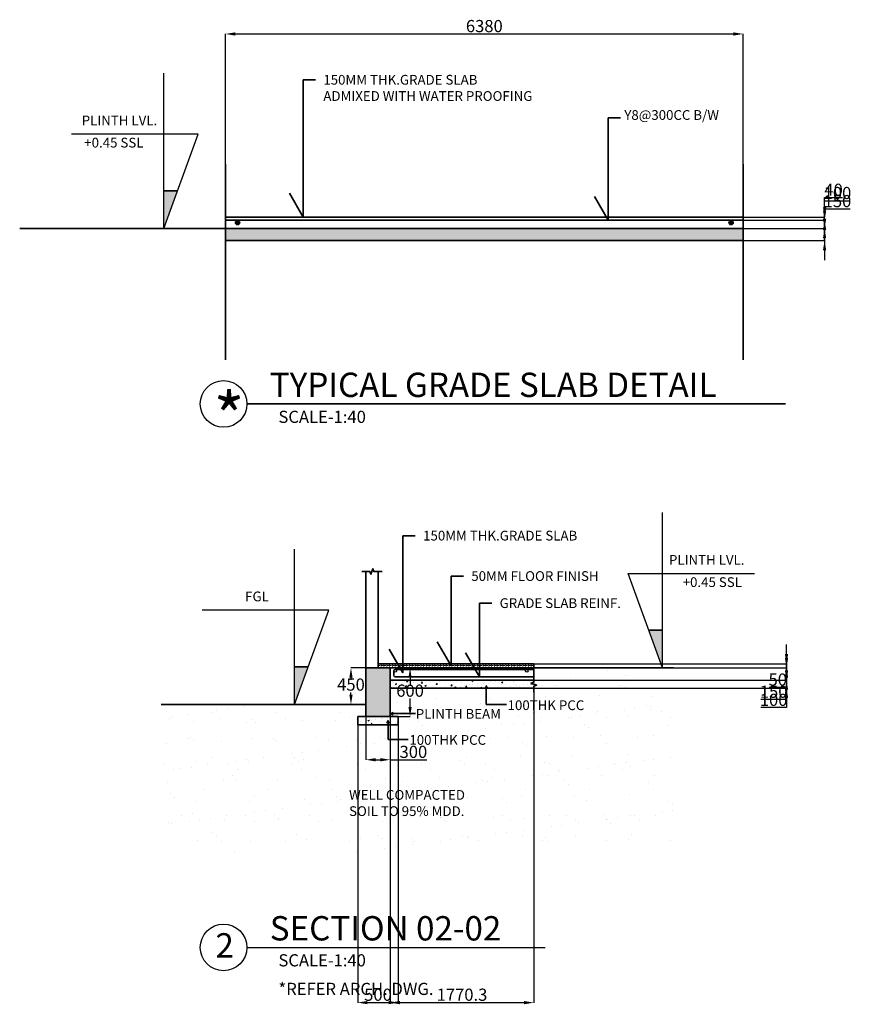
# Model space of a CAD drawing. Units: millimetres. Extents: x -174 to 32373, y 27344 to 53129.
# Tile 7 of 7: x 22126 to 32373, y 39727 to 51861. Entities that reach past the tile are written whole.
import ezdxf

# ---------------------------------------------------------------- set-up
doc = ezdxf.new("R2010")
doc.units = ezdxf.units.MM
doc.header["$LTSCALE"] = 50
for name, color, linetype, lineweight in [('S-ANNO-DIMS', 2, 'Continuous', 18), ('S-ANNO-SYMB', 4, 'Continuous', 25), ('S-ANNO-TEXT', 3, 'Continuous', 18), ('S-DETL', 7, 'Continuous', 35), ('S-PATT', 8, 'Continuous', 13), ('S-REIN', 1, 'Continuous', 25)]:
    doc.layers.add(name, color=color, linetype=linetype, lineweight=lineweight)
doc.styles.get("Standard").update_dxf_attribs({"font": 'arial.ttf'})
doc.dimstyles.new('ISO-25', dxfattribs={"dimtxt": 150, "dimasz": 120, "dimexe": 1.25, "dimexo": 0.625, "dimtad": 1, "dimtih": 1, "dimtoh": 1, "dimdec": 0, "dimtxsty": 'Standard', "dimcen": 2.5, "dimadec": 0, "dimazin": 0, "dimtfac": 1, "dimtdec": 0, "dimtmove": 0, "dimatfit": 3, "dimfxl": 1, "dimarcsym": 0})

# ---------------------------------------------------------------- blocks, each defined once
blk = doc.blocks.new('*D17')
at = {"layer": 'Defpoints', "color": 0, "transparency": 16777216}
for p in [(26391, 43273), (26691, 43273), (26691, 42741)]:
    blk.add_point(p, dxfattribs=at)
at = {"layer": 'S-ANNO-DIMS', "color": 0, "lineweight": -2, "transparency": 16777216}
for p, q in [((26391, 43272), (26391, 42740)), ((26691, 43272), (26691, 42740)), ((26511, 42741), (26571, 42741)), ((26691, 42741), (27143, 42741))]:
    blk.add_line(p, q, dxfattribs=at)
at = {"layer": 'S-ANNO-DIMS', "color": 0, "transparency": 16777216}
for points in [[(26511, 42761), (26511, 42721), (26391, 42741)], [(26571, 42761), (26571, 42721), (26691, 42741)]]:
    blk.add_solid(points, dxfattribs=at)
at = {"layer": 'S-ANNO-DIMS', "color": 0, "transparency": 16777216, "insert": (26977, 42819), "char_height": 150, "attachment_point": 5}
blk.add_mtext('300', dxfattribs=at)
blk = doc.blocks.new('*D18')
at = {"layer": 'Defpoints', "color": 0, "transparency": 16777216}
for p in [(26691, 43873), (26936, 43873), (26691, 43273)]:
    blk.add_point(p, dxfattribs=at)
at = {"layer": 'S-ANNO-DIMS', "color": 0, "lineweight": -2, "transparency": 16777216}
for p, q in [((26692, 43873), (26938, 43873)), ((26936, 43753), (26936, 43650)), ((26936, 43393), (26936, 43496)), ((26692, 43273), (26938, 43273))]:
    blk.add_line(p, q, dxfattribs=at)
at = {"layer": 'S-ANNO-DIMS', "color": 0, "transparency": 16777216}
for points in [[(26916, 43753), (26956, 43753), (26936, 43873)], [(26916, 43393), (26956, 43393), (26936, 43273)]]:
    blk.add_solid(points, dxfattribs=at)
at = {"layer": 'S-ANNO-DIMS', "color": 0, "transparency": 16777216, "insert": (26936, 43573), "char_height": 150, "attachment_point": 5}
blk.add_mtext('600', dxfattribs=at)
blk = doc.blocks.new('*D19')
at = {"layer": 'Defpoints', "color": 0, "transparency": 16777216}
for p in [(26208, 43873), (26391, 43873), (26391, 43423)]:
    blk.add_point(p, dxfattribs=at)
at = {"layer": 'S-ANNO-DIMS', "color": 0, "lineweight": -2, "transparency": 16777216}
for p, q in [((26390, 43873), (26207, 43873)), ((26208, 43753), (26208, 43725)), ((26208, 43543), (26208, 43571)), ((26390, 43423), (26207, 43423))]:
    blk.add_line(p, q, dxfattribs=at)
at = {"layer": 'S-ANNO-DIMS', "color": 0, "transparency": 16777216}
for points in [[(26188, 43753), (26228, 43753), (26208, 43873)], [(26188, 43543), (26228, 43543), (26208, 43423)]]:
    blk.add_solid(points, dxfattribs=at)
at = {"layer": 'S-ANNO-DIMS', "color": 0, "transparency": 16777216, "insert": (26208, 43648), "char_height": 150, "attachment_point": 5}
blk.add_mtext('450', dxfattribs=at)
blk = doc.blocks.new('LEVEL-MARK')
for p, q in [((1136, 0), (1136, 1914)), ((1559, 1162), (0, 1162)), ((1136, 0), (1559, 1162))]:
    blk.add_line(p, q)
blk = doc.blocks.new('SECTION-MARK')
blk.add_line((575, 287), (4248, 287))
blk.add_circle((287, 287), 287)
blk = doc.blocks.new('*D67')
at = {"layer": 'Defpoints', "color": 0, "transparency": 16777216}
for p in [(31041, 51685), (24661, 49429), (31041, 49429)]:
    blk.add_point(p, dxfattribs=at)
at = {"layer": 'S-ANNO-DIMS', "color": 0, "lineweight": -2, "transparency": 16777216}
for p, q in [((24661, 49430), (24661, 51687)), ((24781, 51685), (30921, 51685)), ((31041, 49430), (31041, 51687))]:
    blk.add_line(p, q, dxfattribs=at)
at = {"layer": 'S-ANNO-DIMS', "color": 0, "transparency": 16777216}
for points in [[(24781, 51705), (24781, 51665), (24661, 51685)], [(30921, 51705), (30921, 51665), (31041, 51685)]]:
    blk.add_solid(points, dxfattribs=at)
at = {"layer": 'S-ANNO-DIMS', "color": 0, "transparency": 16777216, "insert": (27851, 51763), "char_height": 150, "attachment_point": 5}
blk.add_mtext('6380', dxfattribs=at)
blk = doc.blocks.new('*D68')
at = {"layer": 'Defpoints', "color": 0, "transparency": 16777216}
for p in [(31041, 49289), (32044, 49289), (31041, 49139)]:
    blk.add_point(p, dxfattribs=at)
at = {"layer": 'S-ANNO-DIMS', "color": 0, "lineweight": -2, "transparency": 16777216}
for p, q in [((32044, 49409), (32044, 49529)), ((32044, 49529), (32361, 49529)), ((31042, 49289), (32045, 49289)), ((32044, 49139), (32044, 49289)), ((31042, 49139), (32045, 49139)), ((32044, 49019), (32044, 48899))]:
    blk.add_line(p, q, dxfattribs=at)
at = {"layer": 'S-ANNO-DIMS', "color": 0, "transparency": 16777216}
for points in [[(32024, 49409), (32064, 49409), (32044, 49289)], [(32024, 49019), (32064, 49019), (32044, 49139)]]:
    blk.add_solid(points, dxfattribs=at)
at = {"layer": 'S-ANNO-DIMS', "color": 0, "transparency": 16777216, "insert": (32203, 49606), "char_height": 150, "attachment_point": 5}
blk.add_mtext('150', dxfattribs=at)
blk = doc.blocks.new('*D69')
at = {"layer": 'Defpoints', "color": 0, "transparency": 16777216}
for p in [(31041, 49389), (32044, 49389), (31041, 49289)]:
    blk.add_point(p, dxfattribs=at)
at = {"layer": 'S-ANNO-DIMS', "color": 0, "lineweight": -2, "transparency": 16777216}
for p, q in [((32044, 49509), (32044, 49629)), ((32044, 49629), (32361, 49629)), ((31042, 49389), (32045, 49389)), ((32044, 49289), (32044, 49389)), ((31042, 49289), (32045, 49289)), ((32044, 49169), (32044, 49049))]:
    blk.add_line(p, q, dxfattribs=at)
at = {"layer": 'S-ANNO-DIMS', "color": 0, "transparency": 16777216}
for points in [[(32024, 49509), (32064, 49509), (32044, 49389)], [(32024, 49169), (32064, 49169), (32044, 49289)]]:
    blk.add_solid(points, dxfattribs=at)
at = {"layer": 'S-ANNO-DIMS', "color": 0, "transparency": 16777216, "insert": (32203, 49706), "char_height": 150, "attachment_point": 5}
blk.add_mtext('100', dxfattribs=at)
blk = doc.blocks.new('*D70')
at = {"layer": 'Defpoints', "color": 0, "transparency": 16777216}
for p in [(31041, 49429), (31041, 49389), (32044, 49429)]:
    blk.add_point(p, dxfattribs=at)
at = {"layer": 'S-ANNO-DIMS', "color": 0, "lineweight": -2, "transparency": 16777216}
for p, q in [((32044, 49549), (32044, 49669)), ((32044, 49669), (32265, 49669)), ((31042, 49429), (32045, 49429)), ((31042, 49389), (32045, 49389)), ((32044, 49389), (32044, 49429)), ((32044, 49269), (32044, 49149))]:
    blk.add_line(p, q, dxfattribs=at)
at = {"layer": 'S-ANNO-DIMS', "color": 0, "transparency": 16777216}
for points in [[(32024, 49549), (32064, 49549), (32044, 49429)], [(32024, 49269), (32064, 49269), (32044, 49389)]]:
    blk.add_solid(points, dxfattribs=at)
at = {"layer": 'S-ANNO-DIMS', "color": 0, "transparency": 16777216, "insert": (32155, 49746), "char_height": 150, "attachment_point": 5}
blk.add_mtext('40', dxfattribs=at)
blk = doc.blocks.new('*D71')
at = {"layer": 'Defpoints', "color": 0, "transparency": 16777216}
for p in [(26691, 43873), (28461, 43923), (31575, 43873)]:
    blk.add_point(p, dxfattribs=at)
at = {"layer": 'S-ANNO-DIMS', "color": 0, "lineweight": -2, "transparency": 16777216}
for p, q in [((31575, 44043), (31575, 44163)), ((26692, 43873), (31576, 43873)), ((28462, 43923), (31576, 43923)), ((31575, 43923), (31575, 43873)), ((31575, 43753), (31575, 43633)), ((31575, 43633), (31360, 43633))]:
    blk.add_line(p, q, dxfattribs=at)
at = {"layer": 'S-ANNO-DIMS', "color": 0, "transparency": 16777216}
for points in [[(31555, 44043), (31595, 44043), (31575, 43923)], [(31555, 43753), (31595, 43753), (31575, 43873)]]:
    blk.add_solid(points, dxfattribs=at)
at = {"layer": 'S-ANNO-DIMS', "color": 0, "transparency": 16777216, "insert": (31467, 43710), "char_height": 150, "attachment_point": 5}
blk.add_mtext('50', dxfattribs=at)
blk = doc.blocks.new('*D72')
at = {"layer": 'Defpoints', "color": 0, "transparency": 16777216}
for p in [(26691, 43873), (28461, 43723), (31575, 43723)]:
    blk.add_point(p, dxfattribs=at)
at = {"layer": 'S-ANNO-DIMS', "color": 0, "lineweight": -2, "transparency": 16777216}
for p, q in [((31575, 43993), (31575, 44113)), ((26692, 43873), (31576, 43873)), ((31575, 43873), (31575, 43723)), ((28462, 43723), (31576, 43723)), ((31575, 43603), (31575, 43483)), ((31575, 43483), (31257, 43483))]:
    blk.add_line(p, q, dxfattribs=at)
at = {"layer": 'S-ANNO-DIMS', "color": 0, "transparency": 16777216}
for points in [[(31555, 43993), (31595, 43993), (31575, 43873)], [(31555, 43603), (31595, 43603), (31575, 43723)]]:
    blk.add_solid(points, dxfattribs=at)
at = {"layer": 'S-ANNO-DIMS', "color": 0, "transparency": 16777216, "insert": (31416, 43560), "char_height": 150, "attachment_point": 5}
blk.add_mtext('150', dxfattribs=at)
blk = doc.blocks.new('*D73')
at = {"layer": 'Defpoints', "color": 0, "transparency": 16777216}
for p in [(28461, 43723), (28461, 43623), (31575, 43623)]:
    blk.add_point(p, dxfattribs=at)
at = {"layer": 'S-ANNO-DIMS', "color": 0, "lineweight": -2, "transparency": 16777216}
for p, q in [((31575, 43843), (31575, 43963)), ((28462, 43723), (31576, 43723)), ((31575, 43723), (31575, 43623)), ((28462, 43623), (31576, 43623)), ((31575, 43503), (31575, 43383)), ((31575, 43383), (31257, 43383))]:
    blk.add_line(p, q, dxfattribs=at)
at = {"layer": 'S-ANNO-DIMS', "color": 0, "transparency": 16777216}
for points in [[(31555, 43843), (31595, 43843), (31575, 43723)], [(31555, 43503), (31595, 43503), (31575, 43623)]]:
    blk.add_solid(points, dxfattribs=at)
at = {"layer": 'S-ANNO-DIMS', "color": 0, "transparency": 16777216, "insert": (31416, 43460), "char_height": 150, "attachment_point": 5}
blk.add_mtext('100', dxfattribs=at)
blk = doc.blocks.new('*D74')
at = {"layer": 'Defpoints', "color": 0, "transparency": 16777216}
for p in [(26691, 43623), (28461, 43623), (28461, 39748)]:
    blk.add_point(p, dxfattribs=at)
at = {"layer": 'S-ANNO-DIMS', "color": 0, "lineweight": -2, "transparency": 16777216}
for p, q in [((26691, 43622), (26691, 39747)), ((28461, 43622), (28461, 39747)), ((26811, 39748), (28341, 39748))]:
    blk.add_line(p, q, dxfattribs=at)
at = {"layer": 'S-ANNO-DIMS', "color": 0, "transparency": 16777216}
for points in [[(26811, 39768), (26811, 39728), (26691, 39748)], [(28341, 39768), (28341, 39728), (28461, 39748)]]:
    blk.add_solid(points, dxfattribs=at)
at = {"layer": 'S-ANNO-DIMS', "color": 0, "transparency": 16777216, "insert": (27576, 39826), "char_height": 150, "attachment_point": 5}
blk.add_mtext('1770.3', dxfattribs=at)
blk = doc.blocks.new('*D75')
at = {"layer": 'Defpoints', "color": 0, "transparency": 16777216}
for p in [(26291, 43173), (26791, 43173), (26791, 39748)]:
    blk.add_point(p, dxfattribs=at)
at = {"layer": 'S-ANNO-DIMS', "color": 0, "lineweight": -2, "transparency": 16777216}
for p, q in [((26291, 43172), (26291, 39747)), ((26791, 43172), (26791, 39747)), ((26411, 39748), (26671, 39748))]:
    blk.add_line(p, q, dxfattribs=at)
at = {"layer": 'S-ANNO-DIMS', "color": 0, "transparency": 16777216}
for points in [[(26411, 39768), (26411, 39728), (26291, 39748)], [(26671, 39768), (26671, 39728), (26791, 39748)]]:
    blk.add_solid(points, dxfattribs=at)
at = {"layer": 'S-ANNO-DIMS', "color": 0, "transparency": 16777216, "insert": (26541, 39826), "char_height": 150, "attachment_point": 5}
blk.add_mtext('500', dxfattribs=at)

msp = doc.modelspace()

# ---------------------------------------------------------------- hatches: boundary and pattern name
at = {"layer": 'S-ANNO-SYMB'}
h = msp.add_hatch(color=256, dxfattribs=at)
h.dxf.hatch_style = 1
h.paths.add_polyline_path([(24070.05, 49753.86), (23900.83, 49753.86), (23900.83, 49288.94)])
h = msp.add_hatch(color=256, dxfattribs=at)
h.dxf.hatch_style = 1
h.paths.add_polyline_path([(30045.84, 44337.76), (29876.62, 44337.76), (30045.84, 43872.85)])
h = msp.add_hatch(color=256, dxfattribs=at)
h.dxf.hatch_style = 1
h.paths.add_polyline_path([(25680.99, 43887.76), (25511.77, 43887.76), (25511.77, 43422.85)])
at = {"layer": 'S-ANNO-TEXT'}
h = msp.add_hatch(color=256, dxfattribs=at)
h.dxf.hatch_style = 1
h.paths.add_polyline_path([(24783.26, 49359.74, 1), (24837.74, 49359.74, 1)])
h = msp.add_hatch(color=256, dxfattribs=at)
h.dxf.hatch_style = 1
h.paths.add_polyline_path([(30864.69, 49359.74, 1), (30919.16, 49359.74, 1)])
h = msp.add_hatch(color=256, dxfattribs=at)
h.dxf.hatch_style = 1
h.paths.add_polyline_path([(27874.75, 43656.98), (27856.42, 43625.22), (27893.08, 43625.22)])
h = msp.add_hatch(color=256, dxfattribs=at)
h.dxf.hatch_style = 1
h.paths.add_polyline_path([(26691.08, 43310.16), (26722.83, 43291.83), (26722.83, 43328.5)])
h = msp.add_hatch(color=256, dxfattribs=at)
h.dxf.hatch_style = 1
h.paths.add_polyline_path([(26664.32, 43229.25), (26645.99, 43197.5), (26682.65, 43197.5)])
at = {"layer": 'S-PATT'}
h = msp.add_hatch(dxfattribs=at)
h.set_pattern_fill('AR-CONC', color=256)
h.paths.add_polyline_path([(31041.22, 49288.94), (24661.21, 49288.94), (24661.21, 49138.94), (31041.22, 49138.94)])
h = msp.add_hatch(dxfattribs=at)
h.set_pattern_fill('AR-SAND', color=256, scale=10)
h.paths.add_polyline_path([(30181.88, 43872.85), (28461.36, 43872.85), (28461.36, 43772.85), (28461.36, 43697.85), (28427.02, 43685.35), (28495.71, 43660.35), (28461.36, 43647.85), (28461.36, 43622.85), (26691.08, 43622.85), (26691.08, 43310.16), (26722.83, 43328.5), (26722.83, 43291.83), (26691.08, 43310.16), (26691.08, 43272.85), (26791.08, 43272.85), (26791.08, 43172.85), (26291.08, 43172.85), (26291.08, 43272.85), (26391.08, 43272.85), (26391.08, 43422.85), (23870.7, 43422.85), (23870.7, 41595.82), (30181.88, 41595.82)])
h.paths.add_polyline_path([(26765.41, 42662.86), (27190.03, 42662.86), (27190.03, 42971.96), (26765.41, 42971.96)], flags=24)
h.paths.add_polyline_path([(26725.13, 43416.91), (27149.75, 43416.91), (27149.75, 43726.02), (26725.13, 43726.02)], flags=24)
h.paths.add_polyline_path([(26146.81, 41978.07), (27786.45, 41978.07), (27786.45, 42427.48), (26146.81, 42427.48)], flags=24)
h.paths.add_polyline_path([(26879.27, 42857.54), (27954.76, 42857.54), (27954.76, 43104.82), (26879.27, 43104.82)], flags=24)
h.paths.add_polyline_path([(26963.84, 43180.72), (28141.66, 43180.72), (28141.66, 43428.01), (26963.84, 43428.01)], flags=24)
h.paths.add_polyline_path([(28089.7, 43285.27), (29165.19, 43285.27), (29165.19, 43532.55), (28089.7, 43532.55)], flags=24)
h = msp.add_hatch(color=256, dxfattribs=at)
h.dxf.hatch_style = 1
h.paths.add_polyline_path([(26391.08, 43272.85), (26691.08, 43272.85), (26691.08, 43872.85), (26391.08, 43872.85)])
h = msp.add_hatch(dxfattribs=at)
h.set_pattern_fill('ANGLE', color=256, scale=5)
h.set_pattern_definition([(0, (0, 0), (0, 34.925), [25.4, -9.525]), (90, (0, 0), (-34.925, 2e-15), [25.4, -9.525])])
h.paths.add_polyline_path([(28461.36, 43872.85), (28461.36, 43922.85), (26541.08, 43922.85), (26541.08, 43872.85), (26691.08, 43872.85)])
h = msp.add_hatch(dxfattribs=at)
h.set_pattern_fill('AR-CONC', color=256)
h.paths.add_polyline_path([(28427.02, 43685.35), (28461.36, 43697.85), (28461.36, 43722.85), (26691.08, 43722.85), (26691.08, 43622.85), (28461.36, 43622.85), (28461.36, 43647.85), (28495.71, 43660.35)])
h = msp.add_hatch(dxfattribs=at)
h.set_pattern_fill('AR-CONC', color=256)
h.paths.add_polyline_path([(26791.08, 43272.85), (26691.08, 43272.85), (26391.08, 43272.85), (26291.08, 43272.85), (26291.08, 43172.85), (26791.08, 43172.85)])

# ---------------------------------------------------------------- linework, layer by layer
at = {"layer": 'S-ANNO-SYMB'}
msp.add_circle((24638.43, 47125.84), 287.47, dxfattribs=at)
at = {"layer": 'S-ANNO-TEXT'}
for points in [[(27874.75, 43656.98), (27856.42, 43625.22), (27893.08, 43625.22)], [(26691.08, 43310.16), (26722.83, 43291.83), (26722.83, 43328.5)], [(26664.32, 43229.25), (26645.99, 43197.5), (26682.65, 43197.5)]]:
    msp.add_lwpolyline(points, close=True, dxfattribs=at)
at = {"layer": 'S-DETL'}
for p, q in [((25618.75, 49428.94), (25618.75, 51119.4)), ((25618.75, 51119.4), (25770.92, 51119.4)), ((29378.5, 49388.94), (29378.5, 50650.37)), ((29378.5, 50650.37), (29530.66, 50650.37)), ((24661.21, 50082.42), (24661.21, 47668.79)), ((31041.22, 50082.42), (31041.22, 47668.79)), ((23900.83, 49753.86), (24070.05, 49753.86)), ((25618.75, 49428.94), (25448.74, 49723.41)), ((29378.5, 49388.94), (29208.48, 49683.41)), ((24661.21, 49428.94), (31041.22, 49428.94)), ((24661.21, 49388.94), (31041.22, 49388.94)), ((22125.72, 49288.94), (31041.22, 49288.94)), ((24661.21, 49138.94), (31041.22, 49138.94)), ((24925.9, 47125.84), (31561.27, 47125.84)), ((26848.57, 43811.37), (26848.57, 45501.83)), ((26848.57, 45501.83), (27000.73, 45501.83)), ((26391.08, 43872.85), (26391.08, 45060.55)), ((26541.08, 43872.85), (26541.08, 45060.55)), ((27442.01, 43899.24), (27442.01, 45003.55)), ((27442.01, 45003.55), (27594.18, 45003.55)), ((27791.08, 43762.85), (27791.08, 44669.94)), ((27791.08, 44669.94), (27943.24, 44669.94)), ((30045.84, 44337.76), (29876.62, 44337.76)), ((27442.01, 43899.24), (27272, 44193.71)), ((26848.57, 43811.37), (26678.56, 44105.84)), ((27791.08, 43762.85), (27621.07, 44057.32)), ((25511.77, 43887.76), (25680.99, 43887.76)), ((26391.08, 43872.85), (26691.08, 43872.85)), ((26391.08, 43272.85), (26391.08, 43872.85)), ((26541.08, 43922.85), (28461.36, 43922.85)), ((26691.08, 43872.85), (26691.08, 43272.85)), ((26691.08, 43872.85), (30181.88, 43872.85)), ((26737.03, 43835.94), (26737.03, 43778.85)), ((26753.03, 43851.94), (28461.36, 43851.94)), ((28461.36, 43922.85), (28461.36, 43772.85)), ((26691.08, 43722.85), (28461.36, 43722.85)), ((26753.03, 43762.85), (28461.36, 43762.85)), ((26691.08, 43622.85), (28461.36, 43622.85)), ((27874.75, 43625.22), (27874.75, 43420.32)), ((23870.7, 43422.85), (26391.08, 43422.85)), ((27874.75, 43420.32), (28124.76, 43420.32)), ((26291.08, 43172.85), (26291.08, 43272.85)), ((26291.08, 43272.85), (26391.08, 43272.85)), ((26691.08, 43272.85), (26391.08, 43272.85)), ((26664.32, 43197.5), (26664.32, 42992.59)), ((26691.08, 43272.85), (26791.08, 43272.85)), ((26722.83, 43310.16), (27002.22, 43310.16)), ((26791.08, 43272.85), (26791.08, 43172.85)), ((26791.08, 43172.85), (26291.08, 43172.85)), ((26664.32, 42992.59), (26914.33, 42992.59))]:
    msp.add_line(p, q, dxfattribs=at)
for points in [[(26341.08, 45060.55), (26441.08, 45060.55), (26453.58, 45026.21), (26478.58, 45094.9), (26491.08, 45060.55), (26591.08, 45060.55)], [(28461.36, 43772.85), (28461.36, 43697.85), (28427.02, 43685.35), (28495.71, 43660.35), (28461.36, 43647.85), (28461.36, 43572.85)]]:
    msp.add_lwpolyline(points, dxfattribs=at)
at = {"layer": 'S-REIN'}
for centre, radius in [((24810.5, 49359.74), 27.24), ((30891.93, 49359.74), 27.24), ((26753.4, 43835.56), 16.38), ((28373.25, 43835.56), 16.38)]:
    msp.add_circle(centre, radius, dxfattribs=at)
for centre, start, end in [((26753.03, 43835.94), 90, 180), ((26753.03, 43778.85), 180, 270)]:
    msp.add_arc(centre, 16, start, end, dxfattribs=at)

# ---------------------------------------------------------------- block references
at = {"layer": 'S-ANNO-SYMB'}
for name, p in [('LEVEL-MARK', (22764.51, 49288.94)), ('LEVEL-MARK', (24375.46, 43422.85)), ('SECTION-MARK', (24350.96, 40140.97))]:
    msp.add_blockref(name, p, dxfattribs=at)
at = {"layer": 'S-ANNO-SYMB', "extrusion": (0, 0, -1), "zscale": -1}
msp.add_blockref('LEVEL-MARK', (-31182.16, 43872.85), dxfattribs=at)

# ---------------------------------------------------------------- texts
at = {"layer": 'S-ANNO-TEXT'}
for s, width, insert, char_height, attachment_point in [('150MM THK.GRADE SLAB\\PADMIXED WITH WATER PROOFING', 2900.7274, (25867.29, 51180.52), 120, 1), ('Y8@300CC B/W', 2900.7274, (29576.25, 50746.47), 120, 1), ('PLINTH LVL.', 1913.0414, (22889.92, 50679.88), 120, 1), ('+0.45 SSL', 1913.0414, (22921.59, 50405.9), 120, 1), ('TYPICAL GRADE SLAB DETAIL', 6501.8432, (25207.44, 47511.38), 300, 1), ('*', 6501.8432, (24514.41, 47259.62), 600, 1), ('SCALE-1:40', 1913.0414, (25314.24, 47041.77), 150, 1), ('150MM THK.GRADE SLAB', 2900.7274, (27097.1, 45562.95), 120, 1), ('PLINTH LVL.', 1913.0414, (31056.75, 45263.78), 120, 3), ('50MM FLOOR FINISH', 2900.7274, (27690.55, 45064.66), 120, 1), ('+0.45 SSL', 1913.0414, (31025.08, 44989.8), 120, 3), ('FGL', 1913.0414, (24903.95, 44813.78), 120, 1), ('GRADE SLAB REINF.', 2900.7274, (28039.62, 44731.06), 120, 1), ('100THK PCC', 1913.0414, (28137.95, 43472.84), 120, 1), ('PLINTH BEAM', 1913.0414, (27006.77, 43366.25), 120, 1), ('100THK PCC', 1913.0414, (26927.52, 43045.11), 120, 1), ('WELL COMPACTED\\PSOIL TO 95% MDD.', 1913.0414, (26184.34, 42367.85), 120, 1), ('SECTION 02-02', 6501.8432, (25207.44, 40813.98), 300, 1), ('2', 6501.8432, (24537.88, 40603.8), 300, 1), ('SCALE-1:40', 1913.0414, (25314.24, 40344.37), 150, 1), ('*REFER ARCH. DWG.', 2642.4337, (25314.24, 39992.18), 150, 1)]:
    msp.add_mtext_dynamic_manual_height_columns(s, width=width, gutter_width=12.5, heights=[0], dxfattribs=dict(at, insert=insert, char_height=char_height, attachment_point=attachment_point))

# ---------------------------------------------------------------- dimensions: what is measured, and where the dimension line sits
at = {"layer": 'S-ANNO-DIMS'}
for base, p1, p2, override, picture, middle in [((31041.22, 51685.41), (24661.21, 49428.94), (31041.22, 49428.94), {"dimdec": 0, "dimlfac": 1, "dimrnd": 0, "dimzin": 0, "dimdsep": 46, "dimlunit": 2}, '*D67', (27851.21, 51762.67)), ((28461.36, 39748.47), (26691.08, 43622.85), (28461.36, 43622.85), {"dimdec": 1, "dimlfac": 1, "dimrnd": 0, "dimzin": 0, "dimdsep": 46, "dimlunit": 2}, '*D74', (27576.22, 39825.73)), ((26691.08, 42741.48), (26391.08, 43272.85), (26691.08, 43272.85), {"dimclrd": 0, "dimclre": 0, "dimclrt": 0}, '*D17', (26977.1, 42818.74)), ((26791.08, 39748.47), (26291.08, 43172.85), (26791.08, 43172.85), {"dimdec": 0, "dimlfac": 1, "dimrnd": 0, "dimzin": 0, "dimdsep": 46, "dimlunit": 2}, '*D75', (26541.08, 39825.68))]:
    dim = msp.add_linear_dim(base=base, p1=p1, p2=p2, dimstyle='ISO-25', override=override, dxfattribs=at)
    dim.commit()
    dim.dimension.update_dxf_attribs({"geometry": picture, "text_midpoint": middle})
for base, p1, p2, override, picture, middle in [((32043.77, 49428.94), (31041.22, 49388.94), (31041.22, 49428.94), {"dimdec": 0, "dimlfac": 1, "dimrnd": 0, "dimzin": 0, "dimdsep": 46, "dimlunit": 2}, '*D70', (32154.6, 49746.15)), ((32043.77, 49388.94), (31041.22, 49288.94), (31041.22, 49388.94), {"dimdec": 0, "dimlfac": 1, "dimrnd": 0, "dimzin": 0, "dimdsep": 46, "dimlunit": 2}, '*D69', (32202.79, 49706.15)), ((32043.77, 49288.94), (31041.22, 49138.94), (31041.22, 49288.94), {"dimdec": 0, "dimlfac": 1, "dimrnd": 0, "dimzin": 0, "dimdsep": 46, "dimlunit": 2}, '*D68', (32202.79, 49606.15)), ((31574.66, 43872.85), (28461.36, 43922.85), (26691.08, 43872.85), {"dimdec": 0, "dimlfac": 1, "dimrnd": 0, "dimzin": 0, "dimdsep": 46, "dimlunit": 2}, '*D71', (31466.85, 43710.06)), ((31574.66, 43722.85), (26691.08, 43872.85), (28461.36, 43722.85), {"dimdec": 0, "dimlfac": 1, "dimrnd": 0, "dimzin": 0, "dimdsep": 46, "dimlunit": 2}, '*D72', (31415.64, 43560.06)), ((31574.66, 43622.85), (28461.36, 43722.85), (28461.36, 43622.85), {"dimdec": 0, "dimlfac": 1, "dimrnd": 0, "dimzin": 0, "dimdsep": 46, "dimlunit": 2}, '*D73', (31415.64, 43460.06)), ((26208.07, 43872.85), (26391.08, 43422.85), (26391.08, 43872.85), {"dimclrd": 0, "dimclre": 0, "dimclrt": 0}, '*D19', (26208.07, 43647.85)), ((26936.36, 43872.85), (26691.08, 43272.85), (26691.08, 43872.85), {"dimclrd": 0, "dimclre": 0, "dimclrt": 0}, '*D18', (26936.36, 43572.85))]:
    dim = msp.add_linear_dim(base=base, p1=p1, p2=p2, angle=90, dimstyle='ISO-25', override=override, dxfattribs=at)
    dim.commit()
    dim.dimension.update_dxf_attribs({"geometry": picture, "text_midpoint": middle})

doc.saveas('drawing.dxf')
